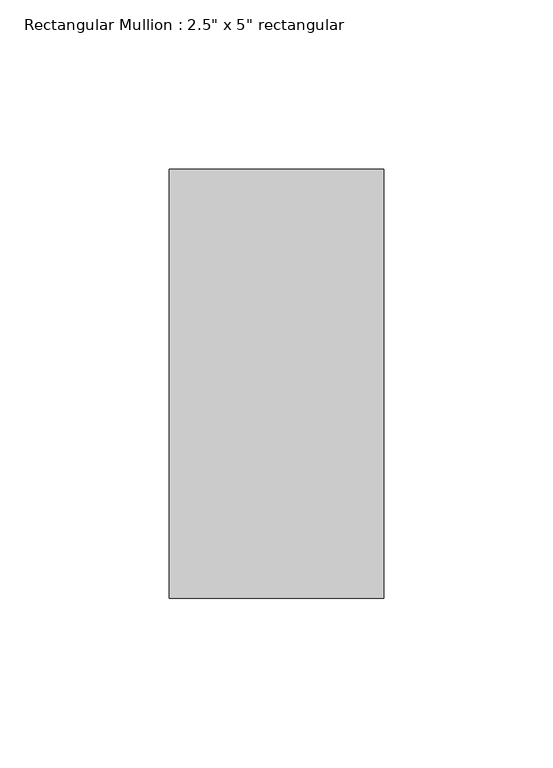
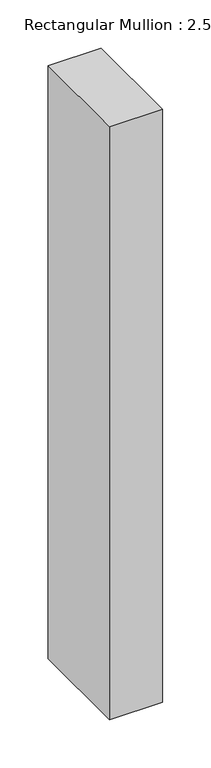
"""IFC4 building model written with IfcOpenShell, lengths in millimetres: member geometry."""

from ifc_helpers import new_model, si_unit, frame, origin, place, context, project, spatial, polyline, outline, extrude, source, transform, mapped, element, save


def member_798d6cad(model_context):
    return source(origin(), model_context, "Body", "SweptSolid", [
        extrude(outline(polyline([(31.75, 63.5), (31.75, -63.5), (-31.75, -63.5), (-31.75, 63.5), (31.75, 63.5)])), frame((0.0, 0.0, -749.3), z_axis=(0.0, 0.0, 1.0), x_axis=(1.0, 0.0, 0.0)), (0.0, 0.0, 1.0), 749.3),
    ])


if __name__ == "__main__":
    model = new_model("IFC4")
    model_context = context("Model", 3, world=origin())
    ifc_project = project(units=[si_unit("LENGTHUNIT", "METRE", prefix="MILLI")], contexts=[model_context])
    site = spatial("IfcSite", under=ifc_project)
    building = spatial("IfcBuilding", under=site)
    placement = place(None, origin())
    member_shape = member_798d6cad(model_context)
    element("IfcMember", 1, ObjectType="Rectangular Mullion : 2.5\" x 5\" rectangular", at=placement, inside=building, context=model_context, shape_type="MappedRepresentation", body=[
        mapped(member_shape, transform((0.0, 0.0, 0.0), x_axis=(1.0, 0.0, 0.0), y_axis=(0.0, 1.0, 0.0), z_axis=(0.0, 0.0, 1.0))),
    ])
    save(model, "model.ifc")

# Revit data of these elements
# Type "Rectangular Mullion : 2.5\" x 5\" rectangular"
#   built-in parameter 1007304 = 0.416667 (stored number, unit not read)
#   built-in parameter 1007301 = 0.104167 (stored number, unit not read)
#   built-in parameter 1007300 = 0.104167 (stored number, unit not read)
